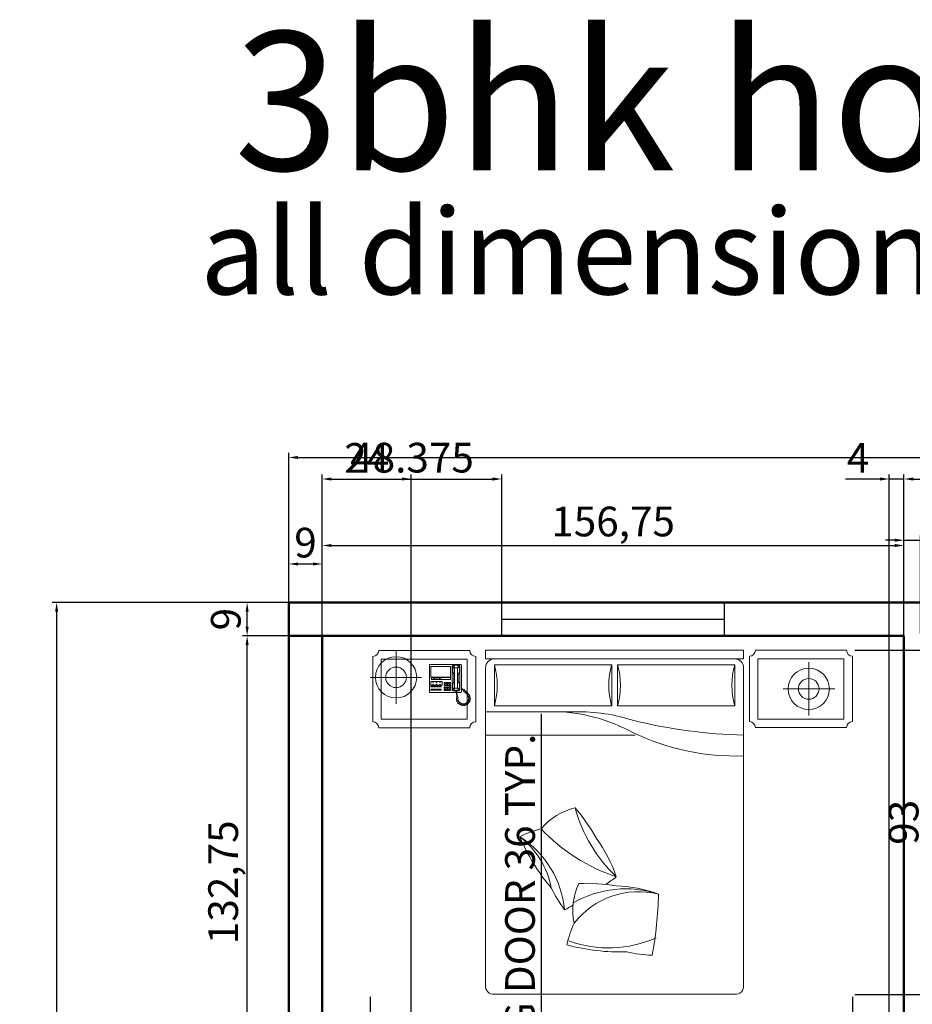
# Model space of a CAD drawing. Units: inches. Extents: x -349 to 9053, y 635 to 6001.
# Tile 5 of 7: x 257 to 498, y 1018 to 1283. Entities that reach past the tile are written whole.
import ezdxf

# ---------------------------------------------------------------- set-up
doc = ezdxf.new("R2010")
doc.units = ezdxf.units.IN
for name, color, linetype, lineweight in [('A-ANNO-DIMS', 2, 'Continuous', 18), ('A-ANNO-TEXT', 7, 'Continuous', 25), ('A-FURN', 8, 'Continuous', 18), ('A-GLAZ', 4, 'Continuous', 25), ('A-WALL', 7, 'Continuous', 50)]:
    doc.layers.add(name, color=color, linetype=linetype, lineweight=lineweight)
doc.styles.get("Standard").update_dxf_attribs({"font": 'arial.ttf'})
doc.dimstyles.new('ISO-25', dxfattribs={"dimtxt": 8, "dimasz": 2.5, "dimexe": 1.25, "dimexo": 0.625, "dimtad": 1, "dimtxsty": 'Standard', "dimcen": 2.5, "dimadec": 0, "dimazin": 0, "dimtfac": 1, "dimtmove": 0, "dimatfit": 3, "dimfxl": 1, "dimarcsym": 0})

# ---------------------------------------------------------------- blocks, each defined once
blk = doc.blocks.new('A$C07097A50')
for p, q in [((0.0153, 1.9631), (0.0153, 1.5831)), ((0.0503, 1.9981), (0.5803, 1.9981)), ((0.0653, 1.9481), (0.0653, 1.5981)), ((0.0653, 1.9481), (0.5653, 1.9481)), ((0.1513, 1.6872), (0.1513, 1.9968)), ((0.5653, 1.9481), (0.5653, 1.5981)), ((0.6153, 1.9631), (0.6153, 1.5831)), ((0.6716, 1.9489), (0.6716, 2.0001)), ((0.6716, 2.0001), (2.1719, 2.0001)), ((2.1719, 1.9489), (0.6716, 1.9489)), ((2.1719, 1.9489), (2.1719, 2.0001)), ((2.2051, 1.9643), (2.2051, 1.5843)), ((2.7701, 1.9993), (2.2401, 1.9993)), ((2.2551, 1.9493), (2.2551, 1.5993)), ((2.7551, 1.9493), (2.2551, 1.9493)), ((2.7551, 1.9493), (2.7551, 1.5993)), ((2.8051, 1.9643), (2.8051, 1.5843)), ((0.3481, 1.9163), (0.3458, 1.914)), ((0.3458, 1.914), (0.3458, 1.7563)), ((0.3481, 1.9163), (0.5287, 1.9163)), ((0.3526, 1.9037), (0.3526, 1.8431)), ((0.4669, 1.9037), (0.3526, 1.9037)), ((0.4669, 1.8431), (0.4669, 1.9037)), ((0.4772, 1.9071), (0.4818, 1.9129)), ((0.4772, 1.7688), (0.4772, 1.9071)), ((0.4818, 1.9094), (0.4807, 1.9049)), ((0.4807, 1.9049), (0.4807, 1.874)), ((0.4807, 1.9049), (0.4909, 1.8946)), ((0.4818, 1.9129), (0.5161, 1.9129)), ((0.4864, 1.9117), (0.4818, 1.9094)), ((0.4921, 1.8969), (0.4864, 1.9117)), ((0.4864, 1.9117), (0.5138, 1.9117)), ((0.4909, 1.8946), (0.4921, 1.8969)), ((0.4909, 1.8431), (0.4909, 1.8946)), ((0.5081, 1.8969), (0.4921, 1.8969)), ((0.5081, 1.8969), (0.5138, 1.9117)), ((0.5092, 1.8946), (0.5081, 1.8969)), ((0.5195, 1.9049), (0.5092, 1.8946)), ((0.5092, 1.8431), (0.5092, 1.8946)), ((0.5138, 1.9117), (0.5184, 1.9094)), ((0.5161, 1.9129), (0.5218, 1.9071)), ((0.5184, 1.9094), (0.5195, 1.9049)), ((0.5195, 1.9049), (0.5195, 1.874)), ((0.5218, 1.9071), (0.5218, 1.77)), ((0.5287, 1.9163), (0.5309, 1.914)), ((0.5309, 1.914), (0.5309, 1.7563)), ((0.6716, 1.8977), (0.6716, 0.0512)), ((2.1719, 0.0512), (2.1719, 1.8977)), ((2.5505, 1.6201), (2.5505, 1.9296)), ((0, 1.8416), (0.3001, 1.8416)), ((0.3526, 1.8431), (0.4669, 1.8431)), ((0.3572, 1.8409), (0.3572, 1.8294)), ((0.4669, 1.8409), (0.3572, 1.8409)), ((0.3664, 1.8409), (0.3664, 1.8294)), ((0.3755, 1.8409), (0.3755, 1.8294)), ((0.3846, 1.8409), (0.3846, 1.8294)), ((0.3938, 1.8409), (0.3938, 1.8294)), ((0.4029, 1.8409), (0.4029, 1.8294)), ((0.4121, 1.8409), (0.4121, 1.8294)), ((0.4669, 1.8294), (0.4669, 1.8409)), ((0.4807, 1.874), (0.4829, 1.8683)), ((0.4829, 1.8683), (0.4864, 1.8626)), ((0.4864, 1.8626), (0.4875, 1.8546)), ((0.4875, 1.8546), (0.4875, 1.8431)), ((0.4875, 1.8214), (0.4875, 1.8431)), ((0.4909, 1.8431), (0.4909, 1.7814)), ((0.5092, 1.8431), (0.5092, 1.7814)), ((0.5138, 1.8626), (0.5127, 1.8546)), ((0.5127, 1.8546), (0.5127, 1.8431)), ((0.5127, 1.8214), (0.5127, 1.8431)), ((0.5172, 1.8683), (0.5138, 1.8626)), ((0.5195, 1.874), (0.5172, 1.8683)), ((0.4201, 1.8168), (0.3526, 1.8168)), ((0.3526, 1.8168), (0.3526, 1.7963)), ((0.3526, 1.7963), (0.4201, 1.7963)), ((0.3652, 1.7906), (0.3538, 1.7906)), ((0.3538, 1.7906), (0.3538, 1.786)), ((0.3538, 1.786), (0.3652, 1.786)), ((0.3572, 1.8294), (0.4669, 1.8294)), ((0.3675, 1.8146), (0.3641, 1.8146)), ((0.3641, 1.8146), (0.3641, 1.8111)), ((0.3641, 1.8111), (0.3675, 1.8111)), ((0.3641, 1.802), (0.3641, 1.7986)), ((0.3675, 1.802), (0.3641, 1.802)), ((0.3641, 1.7986), (0.3675, 1.7986)), ((0.3652, 1.786), (0.3652, 1.7906)), ((0.3675, 1.8111), (0.3675, 1.8146)), ((0.3675, 1.7986), (0.3675, 1.802)), ((0.3812, 1.7906), (0.3698, 1.7906)), ((0.3698, 1.7906), (0.3698, 1.786)), ((0.3698, 1.786), (0.3812, 1.786)), ((0.3812, 1.786), (0.3812, 1.7906)), ((0.3846, 1.8146), (0.3846, 1.8111)), ((0.3881, 1.8146), (0.3846, 1.8146)), ((0.3846, 1.8111), (0.3881, 1.8111)), ((0.3846, 1.802), (0.3846, 1.7986)), ((0.3881, 1.802), (0.3846, 1.802)), ((0.3846, 1.7986), (0.3881, 1.7986)), ((0.3972, 1.7906), (0.3858, 1.7906)), ((0.3858, 1.7906), (0.3858, 1.786)), ((0.3858, 1.786), (0.3972, 1.786)), ((0.3881, 1.8111), (0.3881, 1.8146)), ((0.3881, 1.7986), (0.3881, 1.802)), ((0.3972, 1.786), (0.3972, 1.7906)), ((0.4018, 1.7906), (0.4018, 1.786)), ((0.4132, 1.7906), (0.4018, 1.7906)), ((0.4018, 1.786), (0.4132, 1.786)), ((0.4052, 1.8146), (0.4052, 1.8111)), ((0.4086, 1.8146), (0.4052, 1.8146)), ((0.4052, 1.8111), (0.4086, 1.8111)), ((0.4052, 1.802), (0.4052, 1.7986)), ((0.4086, 1.802), (0.4052, 1.802)), ((0.4052, 1.7986), (0.4086, 1.7986)), ((0.4086, 1.8111), (0.4086, 1.8146)), ((0.4086, 1.7986), (0.4086, 1.802)), ((0.4132, 1.786), (0.4132, 1.7906)), ((0.4201, 1.7963), (0.4201, 1.8168)), ((0.4304, 1.8111), (0.4395, 1.8111)), ((0.4304, 1.8043), (0.4304, 1.8111)), ((0.4395, 1.8043), (0.4304, 1.8043)), ((0.4304, 1.7986), (0.4395, 1.7986)), ((0.4304, 1.7917), (0.4304, 1.7986)), ((0.4395, 1.7917), (0.4304, 1.7917)), ((0.4304, 1.778), (0.4304, 1.7848)), ((0.4304, 1.7848), (0.4395, 1.7848)), ((0.4395, 1.778), (0.4304, 1.778)), ((0.4395, 1.8111), (0.4395, 1.8043)), ((0.4395, 1.7986), (0.4395, 1.7917)), ((0.4395, 1.7848), (0.4395, 1.778)), ((0.4441, 1.8043), (0.4441, 1.8111)), ((0.4441, 1.8111), (0.4532, 1.8111)), ((0.4532, 1.8043), (0.4441, 1.8043)), ((0.4441, 1.7986), (0.4532, 1.7986)), ((0.4441, 1.7917), (0.4441, 1.7986)), ((0.4532, 1.7917), (0.4441, 1.7917)), ((0.4441, 1.778), (0.4441, 1.7848)), ((0.4441, 1.7848), (0.4532, 1.7848)), ((0.4532, 1.778), (0.4441, 1.778)), ((0.4532, 1.8111), (0.4532, 1.8043)), ((0.4532, 1.7986), (0.4532, 1.7917)), ((0.4532, 1.7848), (0.4532, 1.778)), ((0.4578, 1.8111), (0.4669, 1.8111)), ((0.4578, 1.8043), (0.4578, 1.8111)), ((0.4669, 1.8043), (0.4578, 1.8043)), ((0.4578, 1.7986), (0.4669, 1.7986)), ((0.4578, 1.7917), (0.4578, 1.7986)), ((0.4669, 1.7917), (0.4578, 1.7917)), ((0.4578, 1.7791), (0.4578, 1.786)), ((0.4578, 1.786), (0.4669, 1.786)), ((0.4669, 1.7791), (0.4578, 1.7791)), ((0.4669, 1.8111), (0.4669, 1.8043)), ((0.4669, 1.7986), (0.4669, 1.7917)), ((0.4669, 1.786), (0.4669, 1.7791)), ((0.4807, 1.802), (0.4829, 1.8077)), ((0.4807, 1.7711), (0.4807, 1.802)), ((0.4807, 1.7711), (0.4909, 1.7814)), ((0.4829, 1.8077), (0.4864, 1.8134)), ((0.4864, 1.8134), (0.4875, 1.8214)), ((0.4921, 1.7791), (0.4864, 1.7643)), ((0.4909, 1.7814), (0.4921, 1.7791)), ((0.5081, 1.7791), (0.4921, 1.7791)), ((0.5092, 1.7814), (0.5081, 1.7791)), ((0.5081, 1.7791), (0.5138, 1.7643)), ((0.5195, 1.7711), (0.5092, 1.7814)), ((0.5138, 1.8134), (0.5127, 1.8214)), ((0.5172, 1.8077), (0.5138, 1.8134)), ((0.5195, 1.802), (0.5172, 1.8077)), ((0.5195, 1.7711), (0.5195, 1.802)), ((0.5378, 1.7743), (0.5309, 1.7768)), ((0.541, 1.7711), (0.5378, 1.7743)), ((2.7018, 1.7745), (2.4017, 1.7745)), ((0.3458, 1.7563), (0.3481, 1.754)), ((0.5, 1.754), (0.3481, 1.754)), ((0.3538, 1.7666), (0.3538, 1.7734)), ((0.3538, 1.7734), (0.3652, 1.7734)), ((0.3652, 1.7666), (0.3538, 1.7666)), ((0.3652, 1.7734), (0.3652, 1.7666)), ((0.3698, 1.7666), (0.3698, 1.7734)), ((0.3698, 1.7734), (0.3812, 1.7734)), ((0.3812, 1.7666), (0.3698, 1.7666)), ((0.3812, 1.7734), (0.3812, 1.7666)), ((0.3858, 1.7666), (0.3858, 1.7734)), ((0.3858, 1.7734), (0.3972, 1.7734)), ((0.3972, 1.7666), (0.3858, 1.7666)), ((0.3972, 1.7734), (0.3972, 1.7666)), ((0.4018, 1.7734), (0.4132, 1.7734)), ((0.4018, 1.7666), (0.4018, 1.7734)), ((0.4132, 1.7666), (0.4018, 1.7666)), ((0.4132, 1.7734), (0.4132, 1.7666)), ((0.4304, 1.7723), (0.4395, 1.7723)), ((0.4304, 1.7654), (0.4304, 1.7723)), ((0.4395, 1.7654), (0.4304, 1.7654)), ((0.4395, 1.7723), (0.4395, 1.7654)), ((0.4441, 1.7723), (0.4532, 1.7723)), ((0.4441, 1.7654), (0.4441, 1.7723)), ((0.4532, 1.7654), (0.4441, 1.7654)), ((0.4532, 1.7723), (0.4532, 1.7654)), ((0.4578, 1.7654), (0.4578, 1.7723)), ((0.4578, 1.7723), (0.4669, 1.7723)), ((0.4669, 1.7654), (0.4578, 1.7654)), ((0.4669, 1.7723), (0.4669, 1.7654)), ((0.4829, 1.7631), (0.4772, 1.7688)), ((0.4818, 1.7666), (0.4807, 1.7711)), ((0.4864, 1.7643), (0.4818, 1.7666)), ((0.499, 1.7631), (0.4829, 1.7631)), ((0.4864, 1.7643), (0.499, 1.7643)), ((0.5024, 1.7677), (0.4989, 1.7677)), ((0.4989, 1.7677), (0.4991, 1.7578)), ((0.4991, 1.7578), (0.5019, 1.7463)), ((0.5019, 1.7463), (0.5047, 1.7354)), ((0.5026, 1.7254), (0.5021, 1.7199)), ((0.5021, 1.7199), (0.5088, 1.7187)), ((0.5088, 1.7187), (0.5023, 1.7148)), ((0.503, 1.7585), (0.5024, 1.7677)), ((0.5026, 1.7643), (0.5138, 1.7643)), ((0.5051, 1.728), (0.5026, 1.7254)), ((0.5161, 1.7631), (0.5027, 1.7631)), ((0.5047, 1.7511), (0.503, 1.7585)), ((0.5287, 1.754), (0.504, 1.754)), ((0.5047, 1.7354), (0.5044, 1.7294)), ((0.5044, 1.7294), (0.5051, 1.728)), ((0.5074, 1.7403), (0.5047, 1.7511)), ((0.5081, 1.7347), (0.5074, 1.7403)), ((0.5079, 1.7287), (0.5081, 1.7347)), ((0.5121, 1.7257), (0.5079, 1.7287)), ((0.5111, 1.7203), (0.5121, 1.7257)), ((0.5123, 1.7058), (0.5111, 1.7203)), ((0.5138, 1.7643), (0.5184, 1.7666)), ((0.5218, 1.77), (0.5161, 1.7631)), ((0.5184, 1.7666), (0.5195, 1.7711)), ((0.5309, 1.7563), (0.5287, 1.754)), ((0.5309, 1.7723), (0.536, 1.7709)), ((0.536, 1.7709), (0.5406, 1.7672)), ((0.5406, 1.7672), (0.5418, 1.7656)), ((0.5434, 1.7689), (0.541, 1.7711)), ((0.5442, 1.7658), (0.5418, 1.7634)), ((0.5418, 1.7656), (0.5442, 1.7658)), ((0.5418, 1.7634), (0.5511, 1.7552)), ((0.5477, 1.7705), (0.5434, 1.7689)), ((0.5497, 1.7685), (0.5477, 1.7705)), ((0.5481, 1.765), (0.5497, 1.7685)), ((0.5509, 1.7672), (0.5481, 1.765)), ((0.5539, 1.764), (0.5509, 1.7672)), ((0.5511, 1.7552), (0.5662, 1.7423)), ((0.5515, 1.7574), (0.5539, 1.764)), ((0.5577, 1.7606), (0.5515, 1.7574)), ((0.563, 1.7556), (0.5577, 1.7606)), ((0.5618, 1.7483), (0.563, 1.7556)), ((0.567, 1.7515), (0.5618, 1.7483)), ((0.5664, 1.7419), (0.574, 1.7201)), ((0.5714, 1.7469), (0.567, 1.7515)), ((0.5696, 1.7419), (0.5714, 1.7469)), ((0.5766, 1.7426), (0.5697, 1.7419)), ((0.574, 1.7201), (0.5708, 1.7028)), ((0.572, 1.7331), (0.5787, 1.7356)), ((0.5794, 1.7333), (0.572, 1.7331)), ((0.5761, 1.7234), (0.581, 1.728)), ((0.5824, 1.7234), (0.5761, 1.7234)), ((0.5764, 1.7155), (0.5835, 1.7176)), ((0.5787, 1.7356), (0.5766, 1.7426)), ((0.581, 1.728), (0.5794, 1.7333)), ((0.5835, 1.7176), (0.5824, 1.7234)), ((0.5023, 1.7148), (0.5028, 1.7085)), ((0.5028, 1.7085), (0.5102, 1.7078)), ((0.5102, 1.7078), (0.5037, 1.7028)), ((0.5037, 1.7028), (0.5067, 1.6974)), ((0.5067, 1.6974), (0.5137, 1.6988)), ((0.5137, 1.6988), (0.5104, 1.6923)), ((0.5104, 1.6923), (0.5139, 1.6882)), ((0.5211, 1.6947), (0.5123, 1.7058)), ((0.5139, 1.6882), (0.5192, 1.6921)), ((0.5192, 1.6921), (0.5183, 1.6859)), ((0.5183, 1.6859), (0.5227, 1.6831)), ((0.5333, 1.6882), (0.5211, 1.6947)), ((0.5227, 1.6831), (0.5282, 1.6877)), ((0.5282, 1.6877), (0.5276, 1.6801)), ((0.5276, 1.6801), (0.5324, 1.6787)), ((0.5324, 1.6787), (0.5354, 1.6849)), ((0.5472, 1.687), (0.5333, 1.6882)), ((0.5354, 1.6849), (0.5382, 1.6787)), ((0.5382, 1.6787), (0.5421, 1.6782)), ((0.5421, 1.6782), (0.5437, 1.6849)), ((0.5437, 1.6849), (0.5463, 1.6775)), ((0.5463, 1.6775), (0.5507, 1.6787)), ((0.5606, 1.6928), (0.5472, 1.687)), ((0.5507, 1.6787), (0.5509, 1.6849)), ((0.5509, 1.6849), (0.5562, 1.6803)), ((0.5562, 1.6803), (0.5599, 1.6822)), ((0.5592, 1.6891), (0.5641, 1.6831)), ((0.5599, 1.6822), (0.5592, 1.6891)), ((0.5708, 1.7028), (0.5606, 1.6928)), ((0.5641, 1.6831), (0.5678, 1.6863)), ((0.565, 1.6926), (0.5715, 1.6898)), ((0.5678, 1.6863), (0.565, 1.6926)), ((0.5745, 1.6926), (0.5713, 1.6988)), ((0.5713, 1.6988), (0.578, 1.6967)), ((0.5715, 1.6898), (0.5745, 1.6926)), ((0.5743, 1.7076), (0.5814, 1.7074)), ((0.5798, 1.7014), (0.5743, 1.7076)), ((0.5824, 1.712), (0.5764, 1.7155)), ((0.578, 1.6967), (0.5798, 1.7014)), ((0.5814, 1.7074), (0.5824, 1.712)), ((0.0503, 1.5481), (0.5803, 1.5481)), ((0.0653, 1.5981), (0.5653, 1.5981)), ((2.7701, 1.5493), (2.2401, 1.5493)), ((2.7551, 1.5993), (2.2551, 1.5993)), ((0.7228, 0.0001), (2.1207, 0.0001))]:
    blk.add_line(p, q)
at = {"linetype": 'ByBlock'}
for p, q in [((0.7228, 1.6759), (0.7228, 1.9148)), ((0.7228, 1.9148), (1.4047, 1.9148)), ((1.4047, 1.9148), (1.4047, 1.6759)), ((1.4388, 1.6759), (1.4388, 1.9148)), ((1.4388, 1.9148), (2.1207, 1.9148)), ((2.1207, 1.9148), (2.1207, 1.6759)), ((1.4047, 1.6759), (0.7228, 1.6759)), ((2.1207, 1.6759), (1.4388, 1.6759)), ((1.1914, 1.6418), (0.6716, 1.6418)), ((1.5412, 1.5053), (0.6716, 1.5053))]:
    blk.add_line(p, q, dxfattribs=at)
for centre in [(0.1513, 1.8416), (2.5505, 1.7745)]:
    blk.add_circle(centre, 0.12, dxfattribs=at)
for centre in [(0.1513, 1.8416), (2.5505, 1.7745)]:
    blk.add_circle(centre, 0.06)
for centre, radius, start, end in [((0.0153, 1.9981), 0.035, 270, 0), ((0.6153, 1.9981), 0.035, 180, 270), ((0.7228, 1.8977), 0.0512, 90, 180), ((2.1207, 1.8977), 0.0512, 0, 90), ((2.2051, 1.9993), 0.035, 270, 0), ((2.8051, 1.9993), 0.035, 180, 270), ((0.0153, 1.5481), 0.035, 0, 90), ((0.6153, 1.5481), 0.035, 90, 180), ((2.2051, 1.5493), 0.035, 0, 90), ((2.8051, 1.5493), 0.035, 90, 180), ((1.2698, 0.7333), 0.3575, 102.4782, 140.4625), ((0.4476, 0.4335), 0.9879, 28.4971, 41.0566), ((2.0313, 1.3124), 0.8697, 195.336, 226.4193), ((1.1192, 0.4274), 0.548, 103.2034, 117.0362), ((1.7756, 1.7059), 1.0798, 223.6306, 251.4288), ((1.9422, 1.372), 1.1652, 203.0642, 220.3209), ((0.5744, 0.5274), 0.4879, 10.6986, 52.6864), ((0.5678, 0.4375), 0.5655, 5.3391, 57.6895), ((0.6844, 0.4345), 0.7874, 18.3527, 36.6851), ((1.5362, 0.487), 0.3575, 154.0418, 192.0262), ((1.2599, -0.3434), 0.9879, 80.0607, 92.6202), ((0.1017, 2.4319), 2.1977, 305.2966, 307.2418), ((1.4063, -0.1573), 0.7874, 69.9163, 88.2487), ((1.7177, 0.9312), 0.734, 205.259, 216.9351), ((1.4868, 0.0041), 0.6085, 71.81, 120.1351), ((1.5627, 0.1186), 0.4774, 76.1849, 142.0017), ((-0.5205, 0.628), 2.1977, 349.4884, 358.8054), ((0.1017, 2.4319), 2.1977, 297.9248, 299.3793), ((1.6822, 0.1789), 0.548, 154.767, 168.5998), ((1.4539, 1.4107), 1.1652, 254.6278, 271.8845), ((1.3874, 0.9578), 0.6885, 250.2936, 293.6414), ((1.6595, 0.9609), 0.734, 256.8226, 268.4988), ((0.717, 0.0455), 0.0458, 172.7599, 277.2401), ((2.1265, 0.0455), 0.0458, 262.7599, 7.2401)]:
    blk.add_arc(centre, radius, start, end)
for centre, radius, start, end in [((0.3133, 1.7953), 0.4265, 343.7398, 16.2602), ((1.8141, 1.7953), 0.4265, 163.7398, 196.2602), ((1.0294, 1.7953), 0.4265, 343.7398, 16.2602), ((2.5302, 1.7953), 0.4265, 163.7398, 196.2602), ((1.053, 0.6571), 0.9853, 61.4328, 88.1261), ((1.2053, 0.5713), 1.0706, 72.1966, 90.7418), ((2.2595, 4.5996), 3.0955, 256.4201, 268.3789), ((2.1283, 2.7745), 1.3903, 244.2427, 271.7984)]:
    blk.add_arc(centre, radius, start, end, dxfattribs=at)
blk = doc.blocks.new('*D8')
at = {"layer": 'A-ANNO-DIMS', "color": 0, "lineweight": -2, "transparency": 16777216}
for p, q in [((338.38, 1126), (317.52, 1126)), ((318.77, 1119.5), (318.77, 1123.5)), ((338.38, 1117), (317.52, 1117))]:
    blk.add_line(p, q, dxfattribs=at)
at = {"layer": 'A-ANNO-DIMS', "color": 0, "transparency": 16777216}
for points in [[(318.36, 1123.5), (319.19, 1123.5), (318.77, 1126)], [(318.36, 1119.5), (319.19, 1119.5), (318.77, 1117)]]:
    blk.add_solid(points, dxfattribs=at)
at = {"layer": 'Defpoints', "color": 0, "transparency": 16777216}
for p in [(318.77, 1126), (339, 1126), (339, 1117)]:
    blk.add_point(p, dxfattribs=at)
at = {"layer": 'A-ANNO-DIMS', "color": 0, "transparency": 16777216, "insert": (314.06, 1121.5), "char_height": 8, "attachment_point": 5, "rotation": 90}
blk.add_mtext('9', dxfattribs=at)
blk = doc.blocks.new('*D9')
at = {"layer": 'A-ANNO-DIMS', "color": 0, "lineweight": -2, "transparency": 16777216}
for p, q in [((338.38, 1117), (317.52, 1117)), ((318.77, 986.75), (318.77, 1114.5)), ((338.38, 984.25), (317.52, 984.25))]:
    blk.add_line(p, q, dxfattribs=at)
at = {"layer": 'A-ANNO-DIMS', "color": 0, "transparency": 16777216}
for points in [[(318.36, 1114.5), (319.19, 1114.5), (318.77, 1117)], [(318.36, 986.75), (319.19, 986.75), (318.77, 984.25)]]:
    blk.add_solid(points, dxfattribs=at)
at = {"layer": 'Defpoints', "color": 0, "transparency": 16777216}
for p in [(318.77, 1117), (339, 1117), (339, 984.25)]:
    blk.add_point(p, dxfattribs=at)
at = {"layer": 'A-ANNO-DIMS', "color": 0, "transparency": 16777216, "insert": (313.34, 1050.62), "char_height": 8, "attachment_point": 5, "rotation": 90}
blk.add_mtext('132,75', dxfattribs=at)
blk = doc.blocks.new('*D12')
at = {"layer": 'A-ANNO-DIMS', "color": 0, "lineweight": -2, "transparency": 16777216}
for p, q in [((330, 1117.63), (330, 1137.62)), ((332.5, 1136.37), (336.5, 1136.37)), ((339, 1117.63), (339, 1137.62))]:
    blk.add_line(p, q, dxfattribs=at)
at = {"layer": 'A-ANNO-DIMS', "color": 0, "transparency": 16777216}
for points in [[(332.5, 1136.78), (332.5, 1135.95), (330, 1136.37)], [(336.5, 1136.78), (336.5, 1135.95), (339, 1136.37)]]:
    blk.add_solid(points, dxfattribs=at)
at = {"layer": 'Defpoints', "color": 0, "transparency": 16777216}
for p in [(339, 1136.37), (330, 1117), (339, 1117)]:
    blk.add_point(p, dxfattribs=at)
at = {"layer": 'A-ANNO-DIMS', "color": 0, "transparency": 16777216, "insert": (334.5, 1141.08), "char_height": 8, "attachment_point": 5}
blk.add_mtext('9', dxfattribs=at)
blk = doc.blocks.new('*D13')
at = {"layer": 'A-ANNO-DIMS', "color": 0, "lineweight": -2, "transparency": 16777216}
for p, q in [((339, 1126.62), (339, 1142.59)), ((341.5, 1141.34), (493.25, 1141.34)), ((495.75, 1126.62), (495.75, 1142.59))]:
    blk.add_line(p, q, dxfattribs=at)
at = {"layer": 'A-ANNO-DIMS', "color": 0, "transparency": 16777216}
for points in [[(341.5, 1141.75), (341.5, 1140.92), (339, 1141.34)], [(493.25, 1141.75), (493.25, 1140.92), (495.75, 1141.34)]]:
    blk.add_solid(points, dxfattribs=at)
at = {"layer": 'Defpoints', "color": 0, "transparency": 16777216}
for p in [(495.75, 1141.34), (339, 1126), (495.75, 1126)]:
    blk.add_point(p, dxfattribs=at)
at = {"layer": 'A-ANNO-DIMS', "color": 0, "transparency": 16777216, "insert": (417.38, 1146.77), "char_height": 8, "attachment_point": 5}
blk.add_mtext('156,75', dxfattribs=at)
blk = doc.blocks.new('*D14')
at = {"layer": 'A-ANNO-DIMS', "color": 0, "lineweight": -2, "transparency": 16777216}
for p, q in [((495.75, 1117.62), (495.75, 1144.01)), ((500.25, 1117.62), (500.25, 1144.01)), ((493.25, 1142.76), (490.75, 1142.76)), ((495.75, 1142.76), (500.25, 1142.76)), ((502.75, 1142.76), (521.45, 1142.76))]:
    blk.add_line(p, q, dxfattribs=at)
at = {"layer": 'A-ANNO-DIMS', "color": 0, "transparency": 16777216}
for points in [[(493.25, 1143.18), (493.25, 1142.35), (495.75, 1142.76)], [(502.75, 1143.18), (502.75, 1142.35), (500.25, 1142.76)]]:
    blk.add_solid(points, dxfattribs=at)
at = {"layer": 'Defpoints', "color": 0, "transparency": 16777216}
for p in [(500.25, 1142.76), (495.75, 1117), (500.25, 1117)]:
    blk.add_point(p, dxfattribs=at)
at = {"layer": 'A-ANNO-DIMS', "color": 0, "transparency": 16777216, "insert": (513.35, 1148.18), "char_height": 8, "attachment_point": 5}
blk.add_mtext('4,5', dxfattribs=at)
blk = doc.blocks.new('*D19')
at = {"layer": 'A-ANNO-DIMS', "color": 0, "lineweight": -2, "transparency": 16777216}
for p, q in [((330, 1126.62), (330, 1166.31)), ((332.5, 1165.06), (711.5, 1165.06)), ((714, 1126.62), (714, 1166.31))]:
    blk.add_line(p, q, dxfattribs=at)
at = {"layer": 'A-ANNO-DIMS', "color": 0, "transparency": 16777216}
for points in [[(332.5, 1165.47), (332.5, 1164.64), (330, 1165.06)], [(711.5, 1165.47), (711.5, 1164.64), (714, 1165.06)]]:
    blk.add_solid(points, dxfattribs=at)
at = {"layer": 'Defpoints', "color": 0, "transparency": 16777216}
for p in [(714, 1165.06), (330, 1126), (714, 1126)]:
    blk.add_point(p, dxfattribs=at)
at = {"layer": 'A-ANNO-DIMS', "color": 0, "transparency": 16777216, "insert": (522, 1169.77), "char_height": 8, "attachment_point": 5}
blk.add_mtext('384', dxfattribs=at)
blk = doc.blocks.new('*D31')
at = {"layer": 'A-ANNO-DIMS', "color": 0, "lineweight": -2, "transparency": 16777216}
for p, q in [((338.38, 1126), (266.19, 1126)), ((267.44, 1123.5), (267.44, 672.5)), ((338.38, 670), (266.19, 670))]:
    blk.add_line(p, q, dxfattribs=at)
at = {"layer": 'A-ANNO-DIMS', "color": 0, "transparency": 16777216}
for points in [[(267.02, 1123.5), (267.86, 1123.5), (267.44, 1126)], [(267.02, 672.5), (267.86, 672.5), (267.44, 670)]]:
    blk.add_solid(points, dxfattribs=at)
at = {"layer": 'Defpoints', "color": 0, "transparency": 16777216}
for p in [(339, 1126), (267.44, 670), (339, 670)]:
    blk.add_point(p, dxfattribs=at)
at = {"layer": 'A-ANNO-DIMS', "color": 0, "transparency": 16777216, "insert": (262.73, 898), "char_height": 8, "attachment_point": 5, "rotation": 90}
blk.add_mtext('456', dxfattribs=at)
blk = doc.blocks.new('WIN-60IN')
for p, q in [((0, -4.5), (0, 4.5)), ((60, -4.5), (60, 4.5)), ((0, 0), (60, 0))]:
    blk.add_line(p, q)
blk = doc.blocks.new('*D43')
at = {"layer": 'A-ANNO-DIMS', "color": 0, "lineweight": -2, "transparency": 16777216}
for p, q in [((398.1, 975.75), (398.1, 1096.01)), ((402.88, 975.75), (396.85, 975.75)), ((398.1, 942.25), (398.1, 973.25)), ((402.88, 939.75), (396.85, 939.75))]:
    blk.add_line(p, q, dxfattribs=at)
at = {"layer": 'A-ANNO-DIMS', "color": 0, "transparency": 16777216}
for points in [[(397.68, 973.25), (398.52, 973.25), (398.1, 975.75)], [(397.68, 942.25), (398.52, 942.25), (398.1, 939.75)]]:
    blk.add_solid(points, dxfattribs=at)
at = {"layer": 'Defpoints', "color": 0, "transparency": 16777216}
for p in [(398.1, 975.75), (403.5, 975.75), (403.5, 939.75)]:
    blk.add_point(p, dxfattribs=at)
at = {"layer": 'A-ANNO-DIMS', "color": 0, "transparency": 16777216, "insert": (393.33, 1037.13), "char_height": 8, "attachment_point": 5, "rotation": 90}
blk.add_mtext('SWING DOOR 36 TYP.', dxfattribs=at)
blk = doc.blocks.new('*D53')
at = {"layer": 'A-ANNO-DIMS', "color": 0, "lineweight": -2, "transparency": 16777216}
for p, q in [((351.88, 1019.76), (351.88, 999.63)), ((481.9, 1019.76), (481.9, 999.63)), ((354.38, 1000.88), (479.4, 1000.88))]:
    blk.add_line(p, q, dxfattribs=at)
at = {"layer": 'A-ANNO-DIMS', "color": 0, "transparency": 16777216}
for points in [[(354.38, 1001.3), (354.38, 1000.47), (351.88, 1000.88)], [(479.4, 1001.3), (479.4, 1000.47), (481.9, 1000.88)]]:
    blk.add_solid(points, dxfattribs=at)
at = {"layer": 'Defpoints', "color": 0, "transparency": 16777216}
for p in [(351.88, 1020.39), (481.9, 1020.39), (481.9, 1000.88)]:
    blk.add_point(p, dxfattribs=at)
at = {"layer": 'A-ANNO-DIMS', "color": 0, "transparency": 16777216, "insert": (416.89, 1005.65), "char_height": 8, "attachment_point": 5}
blk.add_mtext('BED GROUP A 130', dxfattribs=at)
blk = doc.blocks.new('*D54')
at = {"layer": 'A-ANNO-DIMS', "color": 0, "lineweight": -2, "transparency": 16777216}
for p, q in [((482.52, 1113.17), (502.65, 1113.17)), ((501.4, 1022.89), (501.4, 1110.67)), ((482.52, 1020.39), (502.65, 1020.39))]:
    blk.add_line(p, q, dxfattribs=at)
at = {"layer": 'A-ANNO-DIMS', "color": 0, "transparency": 16777216}
for points in [[(500.98, 1110.67), (501.82, 1110.67), (501.4, 1113.17)], [(500.98, 1022.89), (501.82, 1022.89), (501.4, 1020.39)]]:
    blk.add_solid(points, dxfattribs=at)
at = {"layer": 'Defpoints', "color": 0, "transparency": 16777216}
for p in [(481.9, 1113.17), (501.4, 1113.17), (481.9, 1020.39)]:
    blk.add_point(p, dxfattribs=at)
at = {"layer": 'A-ANNO-DIMS', "color": 0, "transparency": 16777216, "insert": (496.69, 1066.78), "char_height": 8, "attachment_point": 5, "rotation": 90}
blk.add_mtext('93', dxfattribs=at)
blk = doc.blocks.new('*D60')
at = {"layer": 'A-ANNO-DIMS', "color": 0, "lineweight": -2, "transparency": 16777216}
for p, q in [((339, 980.38), (339, 1160.5)), ((341.5, 1159.25), (360.5, 1159.25)), ((363, 980.38), (363, 1160.5))]:
    blk.add_line(p, q, dxfattribs=at)
at = {"layer": 'A-ANNO-DIMS', "color": 0, "transparency": 16777216}
for points in [[(341.5, 1159.67), (341.5, 1158.83), (339, 1159.25)], [(360.5, 1159.67), (360.5, 1158.83), (363, 1159.25)]]:
    blk.add_solid(points, dxfattribs=at)
at = {"layer": 'Defpoints', "color": 0, "transparency": 16777216}
for p in [(363, 1159.25), (339, 979.75), (363, 979.75)]:
    blk.add_point(p, dxfattribs=at)
at = {"layer": 'A-ANNO-DIMS', "color": 0, "transparency": 16777216, "insert": (351, 1163.89), "char_height": 8, "attachment_point": 5}
blk.add_mtext('24', dxfattribs=at)
blk = doc.blocks.new('*D69')
at = {"layer": 'A-ANNO-DIMS', "color": 0, "lineweight": -2, "transparency": 16777216}
for p, q in [((339, 1117.62), (339, 1160.5)), ((341.5, 1159.25), (384.88, 1159.25)), ((387.38, 1117.62), (387.38, 1160.5))]:
    blk.add_line(p, q, dxfattribs=at)
at = {"layer": 'A-ANNO-DIMS', "color": 0, "transparency": 16777216}
for points in [[(341.5, 1159.67), (341.5, 1158.83), (339, 1159.25)], [(384.88, 1159.67), (384.88, 1158.83), (387.38, 1159.25)]]:
    blk.add_solid(points, dxfattribs=at)
at = {"layer": 'Defpoints', "color": 0, "transparency": 16777216}
for p in [(387.38, 1159.25), (339, 1117), (387.38, 1117)]:
    blk.add_point(p, dxfattribs=at)
at = {"layer": 'A-ANNO-DIMS', "color": 0, "transparency": 16777216, "insert": (363.19, 1163.96), "char_height": 8, "attachment_point": 5}
blk.add_mtext('48.375', dxfattribs=at)
blk = doc.blocks.new('*D76')
at = {"layer": 'A-ANNO-DIMS', "color": 0, "lineweight": -2, "transparency": 16777216}
for p, q in [((489.25, 1159.25), (479.97, 1159.25)), ((491.75, 878.37), (491.75, 1160.5)), ((495.75, 1159.25), (491.75, 1159.25)), ((495.75, 878.37), (495.75, 1160.5)), ((498.25, 1159.25), (500.75, 1159.25))]:
    blk.add_line(p, q, dxfattribs=at)
at = {"layer": 'A-ANNO-DIMS', "color": 0, "transparency": 16777216}
for points in [[(489.25, 1159.67), (489.25, 1158.83), (491.75, 1159.25)], [(498.25, 1159.67), (498.25, 1158.83), (495.75, 1159.25)]]:
    blk.add_solid(points, dxfattribs=at)
at = {"layer": 'Defpoints', "color": 0, "transparency": 16777216}
for p in [(491.75, 1159.25), (491.75, 877.75), (495.75, 877.75)]:
    blk.add_point(p, dxfattribs=at)
at = {"layer": 'A-ANNO-DIMS', "color": 0, "transparency": 16777216, "insert": (483.36, 1163.88), "char_height": 8, "attachment_point": 5}
blk.add_mtext('4', dxfattribs=at)

msp = doc.modelspace()

# ---------------------------------------------------------------- linework, layer by layer
at = {"layer": 'A-WALL'}
for p, q in [((714, 1126), (330, 1126)), ((330, 1126), (330, 670)), ((330, 1117), (339, 1117)), ((339, 1117), (339, 984.25)), ((339, 1117), (339, 984.25)), ((339, 1117), (495.75, 1117)), ((495.75, 1117), (339, 1117)), ((495.75, 1117), (495.75, 984.25))]:
    msp.add_line(p, q, dxfattribs=at)

# ---------------------------------------------------------------- block references
at = {"layer": 'A-FURN', "xscale": 46.34965574706475, "yscale": 46.34965574706475, "zscale": 46.34965574706475}
msp.add_blockref('A$C07097A50', (351.8836, 1020.4671), dxfattribs=at)
at = {"layer": 'A-GLAZ'}
msp.add_blockref('WIN-60IN', (387.375, 1121.5), dxfattribs=at)

# ---------------------------------------------------------------- texts
at = {"layer": 'A-ANNO-TEXT'}
for s, height, p in [('3bhk house plan', 37.335229, (315.2717, 1242.4307)), ('all dimensions are in inches', 23.100038, (306.0951, 1208.9899))]:
    msp.add_text(s, height=height, dxfattribs=at).set_placement(p)

# ---------------------------------------------------------------- dimensions: what is measured, and where the dimension line sits
at = {"layer": 'A-ANNO-DIMS'}
for base, p1, p2, override, picture, middle in [((714, 1165.0562), (330, 1126), (714, 1126), {"dimclrd": 0, "dimclre": 0, "dimclrt": 0}, '*D19', (522, 1169.7685)), ((387.375, 1159.25), (339, 1117), (387.375, 1117), {"dimdec": 3, "dimlfac": 1, "dimrnd": 0, "dimzin": 0, "dimdsep": 46, "dimlunit": 2}, '*D69', (363.1875, 1163.9623)), ((363, 1159.25), (339, 979.75), (363, 979.75), {"dimdec": 0, "dimlfac": 1, "dimrnd": 0, "dimzin": 0, "dimdsep": 46, "dimlunit": 2}, '*D60', (351, 1163.8914)), ((491.75, 1159.25), (495.75, 877.75), (491.75, 877.75), {"dimdec": 0, "dimlfac": 1, "dimrnd": 0, "dimzin": 0, "dimdsep": 46, "dimlunit": 2}, '*D76', (483.3583, 1163.875)), ((495.75, 1141.3383), (339, 1126), (495.75, 1126), {"dimclrd": 0, "dimclre": 0, "dimclrt": 0}, '*D13', (417.375, 1146.7709)), ((500.25, 1142.763), (495.75, 1117), (500.25, 1117), {"dimclrd": 0, "dimclre": 0, "dimclrt": 0}, '*D14', (513.3484, 1148.1793)), ((339, 1136.3659), (330, 1117), (339, 1117), {"dimclrd": 0, "dimclre": 0, "dimclrt": 0}, '*D12', (334.5, 1141.0755))]:
    dim = msp.add_linear_dim(base=base, p1=p1, p2=p2, dimstyle='ISO-25', override=override, dxfattribs=at)
    dim.commit()
    dim.dimension.update_dxf_attribs({"geometry": picture, "text_midpoint": middle})
for base, p1, p2, override, picture, middle in [((267.4414, 670), (339, 1126), (339, 670), {"dimclrd": 0, "dimclre": 0, "dimclrt": 0}, '*D31', (262.7318, 898)), ((318.7745, 1126), (339, 1117), (339, 1126), {"dimclrd": 0, "dimclre": 0, "dimclrt": 0}, '*D8', (314.0649, 1121.5)), ((318.7745, 1117), (339, 984.25), (339, 1117), {"dimclrd": 0, "dimclre": 0, "dimclrt": 0}, '*D9', (313.3419, 1050.625)), ((501.4016, 1113.1694), (481.8989, 1020.3874), (481.8989, 1113.1694), {"dimdec": 0, "dimlfac": 1, "dimrnd": 0, "dimzin": 0, "dimdsep": 46, "dimlunit": 2}, '*D54', (496.6893, 1066.7784))]:
    dim = msp.add_linear_dim(base=base, p1=p1, p2=p2, angle=90, dimstyle='ISO-25', override=override, dxfattribs=at)
    dim.commit()
    dim.dimension.update_dxf_attribs({"geometry": picture, "text_midpoint": middle})
dim = msp.add_linear_dim(base=(398.1, 975.75), p1=(403.5, 939.75), p2=(403.5, 975.75), angle=90, text='SWING DOOR <> TYP.', dimstyle='ISO-25', override={"dimdec": 0, "dimlfac": 1, "dimrnd": 0, "dimzin": 0, "dimdsep": 46, "dimlunit": 2}, dxfattribs=at)
dim.commit()
dim.dimension.update_dxf_attribs({"geometry": '*D43', "text_midpoint": (393.3331, 1037.1315)})
dim = msp.add_linear_dim(base=(481.8989, 1000.8847), p1=(351.8813, 1020.3874), p2=(481.8989, 1020.3874), text='BED GROUP A <>', dimstyle='ISO-25', override={"dimdec": 0, "dimlfac": 1, "dimrnd": 0, "dimzin": 0, "dimdsep": 46, "dimlunit": 2}, dxfattribs=at)
dim.commit()
dim.dimension.update_dxf_attribs({"geometry": '*D53', "text_midpoint": (416.8901, 1005.6516)})

doc.saveas('drawing.dxf')
